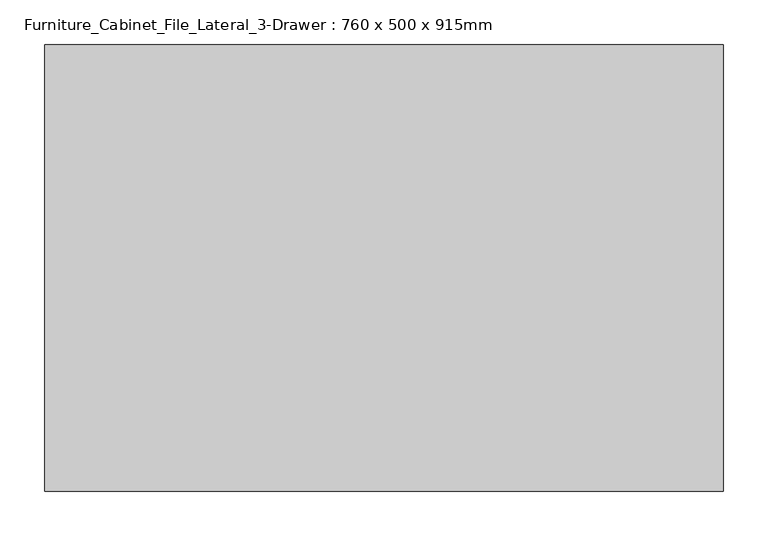
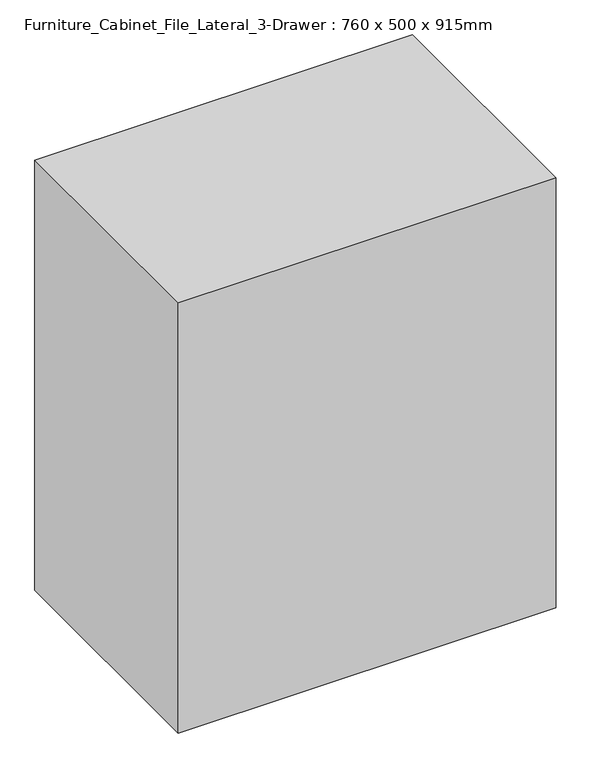
"""IFC4 building model written with IfcOpenShell, lengths in millimetres: furniture geometry, Furniture_Cabinet_File_Lateral_3-Drawer : 760 x 500 x 915mm."""

from ifc_helpers import new_model, si_unit, frame, origin, place, context, project, spatial, polyline, outline, extrude, faceted_brep, source, transform, mapped, element, save


def furniture_cabinet_file_lateral_3_drawer_760_x_500_x_915mm_e725971a(model_context):
    return source(origin(), model_context, "Body", "SolidModel", [
        faceted_brep([(199.9774861, 684.3183761, 915.0), (199.9774861, 1184.3183761, 915.0), (-560.0225139, 1184.3183761, 915.0), (-560.0225139, 684.3183761, 915.0), (199.9774861, 684.3183761, 0.0), (-560.0225139, 684.3183761, 0.0), (-560.0225139, 1184.3183761, 0.0), (199.9774861, 1184.3183761, 0.0), (180.9274861, 1184.3183761, 76.2), (180.9274861, 1184.3183761, 895.95), (-540.9725139, 1184.3183761, 895.95), (-540.9725139, 1184.3183761, 76.2), (-540.9725139, 703.3683761, 76.2), (-540.9725139, 703.3683761, 895.95), (180.9274861, 703.3683761, 895.95), (180.9274861, 703.3683761, 76.2)], [[[0, 1, 2, 3]], [[4, 5, 6, 7]], [[3, 5, 4, 0]], [[2, 6, 5, 3]], [[1, 7, 6, 2], [8, 9, 10, 11]], [[0, 4, 7, 1]], [[12, 13, 14, 15]], [[15, 8, 11, 12]], [[14, 9, 8, 15]], [[13, 10, 9, 14]], [[12, 11, 10, 13]]]),
        extrude(outline(polyline([(895.95, -540.9725139), (622.6999998, -540.9725139), (622.7, 180.9274861), (895.95, 180.9274861), (895.95, -540.9725139)]), holes=[polyline([(686.2, -129.2225139), (648.1, -129.2225139), (648.1, -230.8225139), (686.2, -230.8225139), (686.2, -129.2225139)])]), frame((0.0, 1165.2683761, 0.0), z_axis=(0.0, 1.0, 0.0), x_axis=(0.0, 0.0, 1.0)), (0.0, 0.0, 1.0), 19.05),
        extrude(outline(polyline([(349.45, -540.9725139), (349.45, 180.9274861), (622.7, 180.9274861), (622.6999998, -540.9725139), (349.45, -540.9725139)]), holes=[polyline([(597.3, -129.2225139), (559.2, -129.2225139), (559.2, -230.8225139), (597.3, -230.8225139), (597.3, -129.2225139)])]), frame((0.0, 1165.2683761, 0.0), z_axis=(0.0, 1.0, 0.0), x_axis=(0.0, 0.0, 1.0)), (0.0, 0.0, 1.0), 19.05),
        extrude(outline(polyline([(76.2, -540.9725139), (76.2, 180.9274861), (349.45, 180.9274861), (349.45, -540.9725139), (76.2, -540.9725139)]), holes=[polyline([(324.05, -129.2225139), (285.95, -129.2225139), (285.95, -230.8225139), (324.05, -230.8225139), (324.05, -129.2225139)])]), frame((0.0, 1165.2683761, 0.0), z_axis=(0.0, 1.0, 0.0), x_axis=(0.0, 0.0, 1.0)), (0.0, 0.0, 1.0), 19.05),
    ])


if __name__ == "__main__":
    model = new_model("IFC4")
    model_context = context("Model", 3, world=origin())
    ifc_project = project(units=[si_unit("LENGTHUNIT", "METRE", prefix="MILLI")], contexts=[model_context])
    site = spatial("IfcSite", under=ifc_project)
    building = spatial("IfcBuilding", under=site)
    placement = place(None, origin())
    furniture_cabinet_file_lateral_3_drawer_760_x_500_x_915mm_shape = furniture_cabinet_file_lateral_3_drawer_760_x_500_x_915mm_e725971a(model_context)
    element("IfcFurniture", 1, ObjectType="Furniture_Cabinet_File_Lateral_3-Drawer : 760 x 500 x 915mm", at=placement, inside=building, context=model_context, shape_type="MappedRepresentation", body=[
        mapped(furniture_cabinet_file_lateral_3_drawer_760_x_500_x_915mm_shape, transform((0.0, 0.0, 0.0), x_axis=(1.0, 0.0, 0.0), y_axis=(0.0, 1.0, 0.0), z_axis=(0.0, 0.0, 1.0))),
    ])
    save(model, "model.ifc")

# Revit data of these elements
# Type "Furniture_Cabinet_File_Lateral_3-Drawer : 760 x 500 x 915mm"
#   Keynote = "N"
#   Depth = 1' - 7.68504"
#   Height = 3' - 0.02362"
#   Width = 2' - 5.92126"
#   Material = Metal - Steel
#   Default Elevation = 0
#   Assembly Code = ""
# Element 1 (IfcFurniture, "Furniture_Cabinet_File_Lateral_3-Drawer : 760 x 500 x 915mm")
#   Materials on its faces: "Metal - Steel"
# Materials
#   "Metal - Steel": class "Metal", colour RGB 209 209 209, transparency 0
